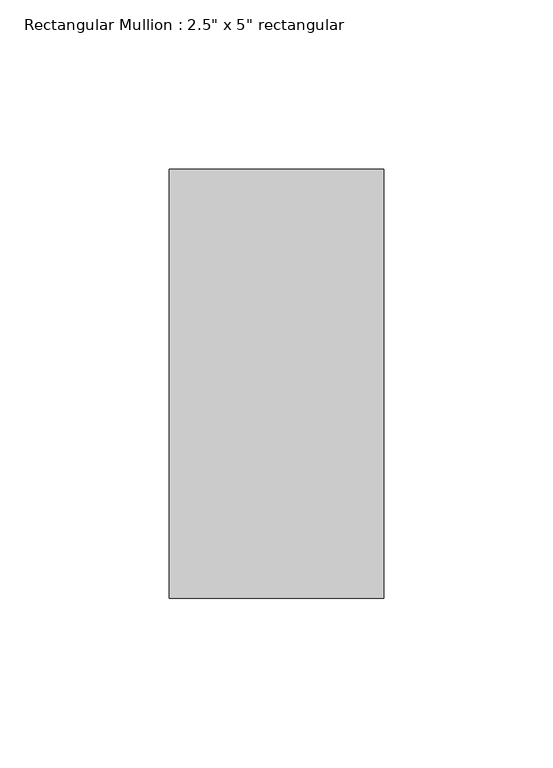
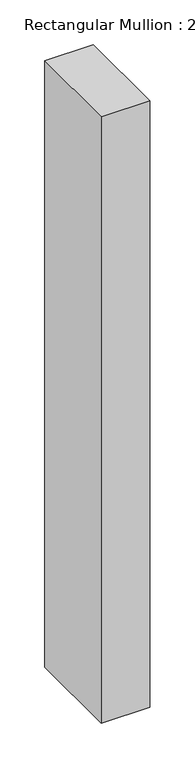
"""IFC4 building model written with IfcOpenShell, lengths in millimetres: member geometry."""

from ifc_helpers import new_model, si_unit, frame, origin, place, context, project, spatial, polyline, outline, extrude, source, transform, mapped, element, save


def member_c5864796(model_context):
    return source(origin(), model_context, "Body", "SweptSolid", [
        extrude(outline(polyline([(0.0, 63.5), (0.0, -63.5), (-63.5, -63.5), (-63.5, 63.5), (0.0, 63.5)])), frame((0.0, 0.0, -831.85), z_axis=(0.0, 0.0, 1.0), x_axis=(1.0, 0.0, 0.0)), (0.0, 0.0, 1.0), 831.85),
    ])


if __name__ == "__main__":
    model = new_model("IFC4")
    model_context = context("Model", 3, world=origin())
    ifc_project = project(units=[si_unit("LENGTHUNIT", "METRE", prefix="MILLI")], contexts=[model_context])
    site = spatial("IfcSite", under=ifc_project)
    building = spatial("IfcBuilding", under=site)
    placement = place(None, origin())
    member_shape = member_c5864796(model_context)
    element("IfcMember", 1, ObjectType="Rectangular Mullion : 2.5\" x 5\" rectangular", at=placement, inside=building, context=model_context, shape_type="MappedRepresentation", body=[
        mapped(member_shape, transform((0.0, 0.0, 0.0), x_axis=(1.0, 0.0, 0.0), y_axis=(0.0, 1.0, 0.0), z_axis=(0.0, 0.0, 1.0))),
    ])
    save(model, "model.ifc")

# Revit data of these elements
# Type "Rectangular Mullion : 2.5\" x 5\" rectangular"
#   built-in parameter 1007304 = 0.416667 (stored number, unit not read)
#   built-in parameter 1007301 = 0.104167 (stored number, unit not read)
#   built-in parameter 1007300 = 0.104167 (stored number, unit not read)
# Element 1 (IfcMember, "Rectangular Mullion : 2.5\" x 5\" rectangular")
#   Materials on its faces: "Aluminum"
# Materials
#   "Aluminum": class "Metal", colour RGB 247 247 247, transparency 0, Description = "Aluminum 6061", Cost = 0
